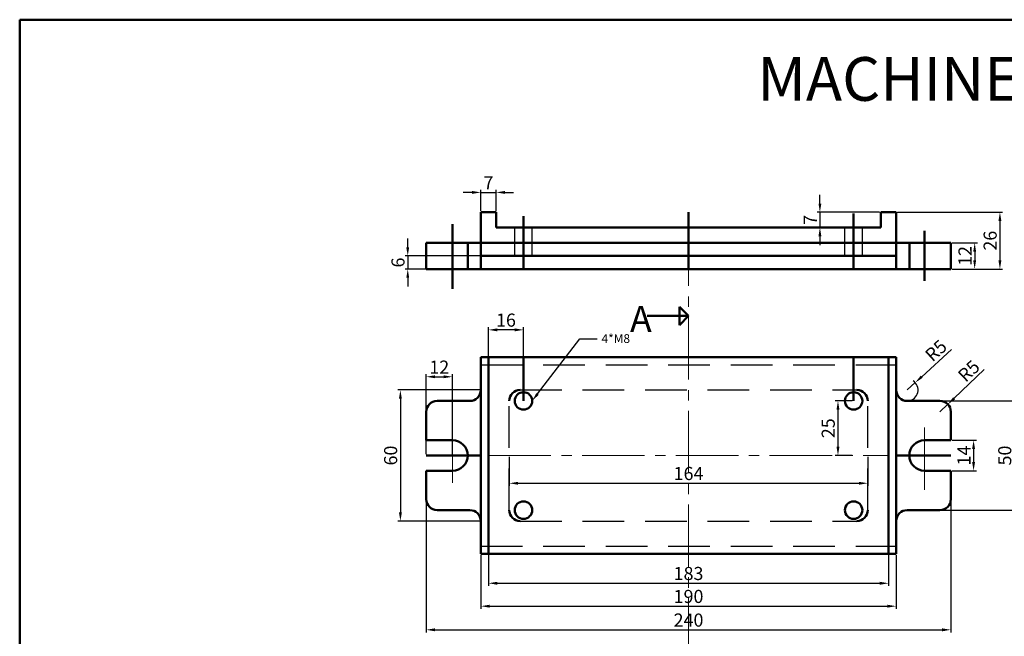
# Model space of a CAD drawing. Units: millimetres. Extents: x -1209 to -333, y 66 to 707.
# Tile 2 of 4: x -1209 to -759, y 424 to 707. Entities that reach past the tile are written whole.
import ezdxf
from ezdxf import colors
from ezdxf.entities.mleader import LeaderData, LeaderLine
from ezdxf.math import Vec2, Vec3

# ---------------------------------------------------------------- set-up
doc = ezdxf.new("R2010")
doc.units = ezdxf.units.MM
doc.header["$LTSCALE"] = 1.5
doc.linetypes.add('CENTER2', pattern=[28.575, 19.05, -3.175, 3.175, -3.175])
doc.linetypes.add('DASHED', pattern=[19.05, 12.7, -6.35])
for name, color, linetype, lineweight in [('M-CNTR', 1, 'CENTER2', 18), ('M-DIMS', 2, 'Continuous', 25), ('M-HIDN', 4, 'DASHED', 25), ('M-OUTL', 7, 'Continuous', 50), ('M-TEXT', 3, 'Continuous', 25), ('M-TTLB', 7, 'Continuous', 50)]:
    doc.layers.add(name, color=color, linetype=linetype, lineweight=lineweight)
doc.styles.get("Standard").update_dxf_attribs({"font": 'arial.ttf'})
doc.dimstyles.new('ISO-25', dxfattribs={"dimtxt": 6, "dimasz": 4, "dimexe": 1.25, "dimexo": 0.625, "dimtad": 1, "dimdec": 0, "dimtxsty": 'Standard', "dimcen": 2.5, "dimadec": 0, "dimazin": 0, "dimtfac": 1, "dimtdec": 0, "dimtmove": 0, "dimatfit": 3, "dimfxl": 1, "dimarcsym": 0})

# ---------------------------------------------------------------- blocks, each defined once
blk = doc.blocks.new('*D1')
at = {"layer": 'Defpoints', "color": 0, "transparency": 16777216}
for p in [(-998.18, 462.21), (-808.18, 462.21), (-808.18, 438.24)]:
    blk.add_point(p, dxfattribs=at)
at = {"layer": 'M-DIMS', "color": 0, "lineweight": -2, "transparency": 16777216}
for p, q in [((-998.18, 461.59), (-998.18, 436.99)), ((-808.18, 461.59), (-808.18, 436.99)), ((-994.18, 438.24), (-812.18, 438.24))]:
    blk.add_line(p, q, dxfattribs=at)
at = {"layer": 'M-DIMS', "color": 0, "transparency": 16777216}
for points in [[(-994.18, 438.9), (-994.18, 437.57), (-998.18, 438.24)], [(-812.18, 438.9), (-812.18, 437.57), (-808.18, 438.24)]]:
    blk.add_solid(points, dxfattribs=at)
at = {"layer": 'M-DIMS', "color": 0, "transparency": 16777216, "insert": (-903.18, 441.93), "char_height": 6, "attachment_point": 5}
blk.add_mtext('190', dxfattribs=at)
blk = doc.blocks.new('*D2')
at = {"layer": 'Defpoints', "color": 0, "transparency": 16777216}
for p in [(-994.68, 465.71), (-811.68, 465.71), (-811.68, 448.73)]:
    blk.add_point(p, dxfattribs=at)
at = {"layer": 'M-DIMS', "color": 0, "lineweight": -2, "transparency": 16777216}
for p, q in [((-994.68, 465.09), (-994.68, 447.48)), ((-811.68, 465.09), (-811.68, 447.48)), ((-990.68, 448.73), (-815.68, 448.73))]:
    blk.add_line(p, q, dxfattribs=at)
at = {"layer": 'M-DIMS', "color": 0, "transparency": 16777216}
for points in [[(-990.68, 449.39), (-990.68, 448.06), (-994.68, 448.73)], [(-815.68, 449.39), (-815.68, 448.06), (-811.68, 448.73)]]:
    blk.add_solid(points, dxfattribs=at)
at = {"layer": 'M-DIMS', "color": 0, "transparency": 16777216, "insert": (-903.18, 452.42), "char_height": 6, "attachment_point": 5}
blk.add_mtext('183', dxfattribs=at)
blk = doc.blocks.new('*D3')
at = {"layer": 'Defpoints', "color": 0, "transparency": 16777216}
for p in [(-1023.18, 487.21), (-783.18, 487.21), (-783.18, 427.42)]:
    blk.add_point(p, dxfattribs=at)
at = {"layer": 'M-DIMS', "color": 0, "lineweight": -2, "transparency": 16777216}
for p, q in [((-1023.18, 486.59), (-1023.18, 426.17)), ((-783.18, 486.59), (-783.18, 426.17)), ((-1019.18, 427.42), (-787.18, 427.42))]:
    blk.add_line(p, q, dxfattribs=at)
at = {"layer": 'M-DIMS', "color": 0, "transparency": 16777216}
for points in [[(-1019.18, 428.09), (-1019.18, 426.75), (-1023.18, 427.42)], [(-787.18, 428.09), (-787.18, 426.75), (-783.18, 427.42)]]:
    blk.add_solid(points, dxfattribs=at)
at = {"layer": 'M-DIMS', "color": 0, "transparency": 16777216, "insert": (-903.18, 431.11), "char_height": 6, "attachment_point": 5}
blk.add_mtext('240', dxfattribs=at)
blk = doc.blocks.new('*D4')
at = {"layer": 'Defpoints', "color": 0, "transparency": 16777216}
for p in [(-998.18, 537.21), (-1034.96, 477.21), (-998.18, 477.21)]:
    blk.add_point(p, dxfattribs=at)
at = {"layer": 'M-DIMS', "color": 0, "lineweight": -2, "transparency": 16777216}
for p, q in [((-998.81, 537.21), (-1036.21, 537.21)), ((-1034.96, 533.21), (-1034.96, 481.21)), ((-998.81, 477.21), (-1036.21, 477.21))]:
    blk.add_line(p, q, dxfattribs=at)
at = {"layer": 'M-DIMS', "color": 0, "transparency": 16777216}
for points in [[(-1035.62, 533.21), (-1034.29, 533.21), (-1034.96, 537.21)], [(-1035.62, 481.21), (-1034.29, 481.21), (-1034.96, 477.21)]]:
    blk.add_solid(points, dxfattribs=at)
at = {"layer": 'M-DIMS', "color": 0, "transparency": 16777216, "insert": (-1038.65, 507.21), "char_height": 6, "attachment_point": 5, "rotation": 90}
blk.add_mtext('60', dxfattribs=at)
blk = doc.blocks.new('*D5')
at = {"layer": 'Defpoints', "color": 0, "transparency": 16777216}
for p in [(-788.18, 532.21), (-788.18, 482.21), (-754.08, 482.21)]:
    blk.add_point(p, dxfattribs=at)
at = {"layer": 'M-DIMS', "color": 0, "lineweight": -2, "transparency": 16777216}
for p, q in [((-787.56, 532.21), (-752.83, 532.21)), ((-754.08, 528.21), (-754.08, 486.21)), ((-787.56, 482.21), (-752.83, 482.21))]:
    blk.add_line(p, q, dxfattribs=at)
at = {"layer": 'M-DIMS', "color": 0, "transparency": 16777216}
for points in [[(-754.75, 528.21), (-753.41, 528.21), (-754.08, 532.21)], [(-754.75, 486.21), (-753.41, 486.21), (-754.08, 482.21)]]:
    blk.add_solid(points, dxfattribs=at)
at = {"layer": 'M-DIMS', "color": 0, "transparency": 16777216, "insert": (-757.77, 507.21), "char_height": 6, "attachment_point": 5, "rotation": 90}
blk.add_mtext('50', dxfattribs=at)
blk = doc.blocks.new('*D6')
at = {"layer": 'Defpoints', "color": 0, "transparency": 16777216}
for p in [(-783.18, 514.21), (-783.18, 500.21), (-772.79, 500.21)]:
    blk.add_point(p, dxfattribs=at)
at = {"layer": 'M-DIMS', "color": 0, "lineweight": -2, "transparency": 16777216}
for p, q in [((-782.56, 514.21), (-771.54, 514.21)), ((-772.79, 510.21), (-772.79, 504.21)), ((-782.56, 500.21), (-771.54, 500.21))]:
    blk.add_line(p, q, dxfattribs=at)
at = {"layer": 'M-DIMS', "color": 0, "transparency": 16777216}
for points in [[(-773.46, 510.21), (-772.13, 510.21), (-772.79, 514.21)], [(-773.46, 504.21), (-772.13, 504.21), (-772.79, 500.21)]]:
    blk.add_solid(points, dxfattribs=at)
at = {"layer": 'M-DIMS', "color": 0, "transparency": 16777216, "insert": (-776.43, 507.21), "char_height": 6, "attachment_point": 5, "rotation": 90}
blk.add_mtext('14', dxfattribs=at)
blk = doc.blocks.new('*D7')
at = {"layer": 'Defpoints', "color": 0, "transparency": 16777216}
for p in [(-788.18, 527.21), (-784.56, 530.66)]:
    blk.add_point(p, dxfattribs=at)
at = {"layer": 'M-DIMS', "color": 0, "lineweight": -2, "transparency": 16777216}
for p, q in [((-767.92, 546.52), (-781.67, 533.42)), ((-788.18, 527.21), (-784.56, 530.66))]:
    blk.add_line(p, q, dxfattribs=at)
at = {"layer": 'M-DIMS', "color": 0, "transparency": 16777216}
blk.add_solid([(-782.13, 533.9), (-781.21, 532.94), (-784.56, 530.66)], dxfattribs=at)
at = {"layer": 'M-DIMS', "color": 0, "transparency": 16777216, "insert": (-774.43, 545.39), "char_height": 6, "attachment_point": 5, "rotation": 43.6176}
blk.add_mtext('R5', dxfattribs=at)
blk = doc.blocks.new('*D8')
at = {"layer": 'Defpoints', "color": 0, "transparency": 16777216}
for p in [(-799.49, 540.58), (-803.18, 537.21)]:
    blk.add_point(p, dxfattribs=at)
at = {"layer": 'M-DIMS', "color": 0, "lineweight": -2, "transparency": 16777216}
for p, q in [((-782.95, 555.67), (-796.53, 543.28)), ((-803.18, 537.21), (-799.49, 540.58))]:
    blk.add_line(p, q, dxfattribs=at)
blk.add_arc((-803.18, 537.21), 5, 277.162, 56.6885, dxfattribs=at)
at = {"layer": 'M-DIMS', "color": 0, "transparency": 16777216}
blk.add_solid([(-796.98, 543.77), (-796.08, 542.78), (-799.49, 540.58)], dxfattribs=at)
at = {"layer": 'M-DIMS', "color": 0, "transparency": 16777216, "insert": (-789.48, 554.69), "char_height": 6, "attachment_point": 5, "rotation": 42.3646}
blk.add_mtext('R5', dxfattribs=at)
blk = doc.blocks.new('*D9')
at = {"layer": 'Defpoints', "color": 0, "transparency": 16777216}
for p in [(-827.68, 532.21), (-834.82, 507.21), (-827.68, 507.21)]:
    blk.add_point(p, dxfattribs=at)
at = {"layer": 'M-DIMS', "color": 0, "lineweight": -2, "transparency": 16777216}
for p, q in [((-828.31, 532.21), (-836.07, 532.21)), ((-834.82, 528.21), (-834.82, 511.21)), ((-828.31, 507.21), (-836.07, 507.21))]:
    blk.add_line(p, q, dxfattribs=at)
at = {"layer": 'M-DIMS', "color": 0, "transparency": 16777216}
for points in [[(-835.49, 528.21), (-834.16, 528.21), (-834.82, 532.21)], [(-835.49, 511.21), (-834.16, 511.21), (-834.82, 507.21)]]:
    blk.add_solid(points, dxfattribs=at)
at = {"layer": 'M-DIMS', "color": 0, "transparency": 16777216, "insert": (-838.51, 519.71), "char_height": 6, "attachment_point": 5, "rotation": 90}
blk.add_mtext('25', dxfattribs=at)
blk = doc.blocks.new('*D10')
at = {"layer": 'Defpoints', "color": 0, "transparency": 16777216}
for p in [(-985.18, 507.21), (-821.18, 507.21), (-821.18, 494.51)]:
    blk.add_point(p, dxfattribs=at)
at = {"layer": 'M-DIMS', "color": 0, "lineweight": -2, "transparency": 16777216}
for p, q in [((-985.18, 506.59), (-985.18, 493.26)), ((-821.18, 506.59), (-821.18, 493.26)), ((-981.18, 494.51), (-825.18, 494.51))]:
    blk.add_line(p, q, dxfattribs=at)
at = {"layer": 'M-DIMS', "color": 0, "transparency": 16777216}
for points in [[(-981.18, 495.17), (-981.18, 493.84), (-985.18, 494.51)], [(-825.18, 495.17), (-825.18, 493.84), (-821.18, 494.51)]]:
    blk.add_solid(points, dxfattribs=at)
at = {"layer": 'M-DIMS', "color": 0, "transparency": 16777216, "insert": (-903.18, 498.19), "char_height": 6, "attachment_point": 5}
blk.add_mtext('164', dxfattribs=at)
blk = doc.blocks.new('*D11')
at = {"layer": 'Defpoints', "color": 0, "transparency": 16777216}
for p in [(-1011.18, 543.26), (-1023.18, 507.21), (-1011.18, 507.21)]:
    blk.add_point(p, dxfattribs=at)
at = {"layer": 'M-DIMS', "color": 0, "lineweight": -2, "transparency": 16777216}
for p, q in [((-1023.18, 507.84), (-1023.18, 544.51)), ((-1019.18, 543.26), (-1015.18, 543.26)), ((-1011.18, 507.84), (-1011.18, 544.51))]:
    blk.add_line(p, q, dxfattribs=at)
at = {"layer": 'M-DIMS', "color": 0, "transparency": 16777216}
for points in [[(-1019.18, 543.92), (-1019.18, 542.59), (-1023.18, 543.26)], [(-1015.18, 543.92), (-1015.18, 542.59), (-1011.18, 543.26)]]:
    blk.add_solid(points, dxfattribs=at)
at = {"layer": 'M-DIMS', "color": 0, "transparency": 16777216, "insert": (-1017.18, 546.89), "char_height": 6, "attachment_point": 5}
blk.add_mtext('12', dxfattribs=at)
blk = doc.blocks.new('*D12')
at = {"layer": 'Defpoints', "color": 0, "transparency": 16777216}
for p in [(-994.68, 564.73), (-994.68, 532.21), (-978.68, 532.21)]:
    blk.add_point(p, dxfattribs=at)
at = {"layer": 'M-DIMS', "color": 0, "lineweight": -2, "transparency": 16777216}
for p, q in [((-994.68, 532.84), (-994.68, 565.98)), ((-982.68, 564.73), (-990.68, 564.73)), ((-978.68, 532.84), (-978.68, 565.98))]:
    blk.add_line(p, q, dxfattribs=at)
at = {"layer": 'M-DIMS', "color": 0, "transparency": 16777216}
for points in [[(-990.68, 565.4), (-990.68, 564.07), (-994.68, 564.73)], [(-982.68, 565.4), (-982.68, 564.07), (-978.68, 564.73)]]:
    blk.add_solid(points, dxfattribs=at)
at = {"layer": 'M-DIMS', "color": 0, "transparency": 16777216, "insert": (-986.68, 568.42), "char_height": 6, "attachment_point": 5}
blk.add_mtext('16', dxfattribs=at)
blk = doc.blocks.new('*D13')
at = {"layer": 'Defpoints', "color": 0, "transparency": 16777216}
for p in [(-783.18, 604.56), (-783.18, 592.56), (-772.3, 592.56)]:
    blk.add_point(p, dxfattribs=at)
at = {"layer": 'M-DIMS', "color": 0, "lineweight": -2, "transparency": 16777216}
for p, q in [((-782.56, 604.56), (-771.05, 604.56)), ((-772.3, 600.56), (-772.3, 596.56)), ((-782.56, 592.56), (-771.05, 592.56))]:
    blk.add_line(p, q, dxfattribs=at)
at = {"layer": 'M-DIMS', "color": 0, "transparency": 16777216}
for points in [[(-772.97, 600.56), (-771.64, 600.56), (-772.3, 604.56)], [(-772.97, 596.56), (-771.64, 596.56), (-772.3, 592.56)]]:
    blk.add_solid(points, dxfattribs=at)
at = {"layer": 'M-DIMS', "color": 0, "transparency": 16777216, "insert": (-775.94, 598.56), "char_height": 6, "attachment_point": 5, "rotation": 90}
blk.add_mtext('12', dxfattribs=at)
blk = doc.blocks.new('*D14')
at = {"layer": 'Defpoints', "color": 0, "transparency": 16777216}
for p in [(-808.18, 618.56), (-783.18, 592.56), (-760.75, 592.56)]:
    blk.add_point(p, dxfattribs=at)
at = {"layer": 'M-DIMS', "color": 0, "lineweight": -2, "transparency": 16777216}
for p, q in [((-807.56, 618.56), (-759.5, 618.56)), ((-760.75, 614.56), (-760.75, 596.56)), ((-782.56, 592.56), (-759.5, 592.56))]:
    blk.add_line(p, q, dxfattribs=at)
at = {"layer": 'M-DIMS', "color": 0, "transparency": 16777216}
for points in [[(-761.42, 614.56), (-760.08, 614.56), (-760.75, 618.56)], [(-761.42, 596.56), (-760.08, 596.56), (-760.75, 592.56)]]:
    blk.add_solid(points, dxfattribs=at)
at = {"layer": 'M-DIMS', "color": 0, "transparency": 16777216, "insert": (-764.44, 605.56), "char_height": 6, "attachment_point": 5, "rotation": 90}
blk.add_mtext('26', dxfattribs=at)
blk = doc.blocks.new('*D15')
at = {"layer": 'Defpoints', "color": 0, "transparency": 16777216}
for p in [(-815.16, 618.56), (-843.09, 611.56), (-815.16, 611.56)]:
    blk.add_point(p, dxfattribs=at)
at = {"layer": 'M-DIMS', "color": 0, "lineweight": -2, "transparency": 16777216}
for p, q in [((-843.09, 622.56), (-843.09, 626.56)), ((-815.78, 618.56), (-844.34, 618.56)), ((-843.09, 618.56), (-843.09, 611.56)), ((-815.78, 611.56), (-844.34, 611.56)), ((-843.09, 607.56), (-843.09, 603.56))]:
    blk.add_line(p, q, dxfattribs=at)
at = {"layer": 'M-DIMS', "color": 0, "transparency": 16777216}
for points in [[(-843.75, 622.56), (-842.42, 622.56), (-843.09, 618.56)], [(-843.75, 607.56), (-842.42, 607.56), (-843.09, 611.56)]]:
    blk.add_solid(points, dxfattribs=at)
at = {"layer": 'M-DIMS', "color": 0, "transparency": 16777216, "insert": (-846.71, 615.06), "char_height": 6, "attachment_point": 5, "rotation": 90}
blk.add_mtext('7', dxfattribs=at)
blk = doc.blocks.new('*D16')
at = {"layer": 'Defpoints', "color": 0, "transparency": 16777216}
for p in [(-991.18, 627.65), (-998.18, 618.56), (-991.18, 618.56)]:
    blk.add_point(p, dxfattribs=at)
at = {"layer": 'M-DIMS', "color": 0, "lineweight": -2, "transparency": 16777216}
for p, q in [((-1002.18, 627.65), (-1006.18, 627.65)), ((-998.18, 619.19), (-998.18, 628.9)), ((-998.18, 627.65), (-991.18, 627.65)), ((-991.18, 619.19), (-991.18, 628.9)), ((-987.18, 627.65), (-983.18, 627.65))]:
    blk.add_line(p, q, dxfattribs=at)
at = {"layer": 'M-DIMS', "color": 0, "transparency": 16777216}
for points in [[(-1002.18, 628.31), (-1002.18, 626.98), (-998.18, 627.65)], [(-987.18, 628.31), (-987.18, 626.98), (-991.18, 627.65)]]:
    blk.add_solid(points, dxfattribs=at)
at = {"layer": 'M-DIMS', "color": 0, "transparency": 16777216, "insert": (-994.68, 631.27), "char_height": 6, "attachment_point": 5}
blk.add_mtext('7', dxfattribs=at)
blk = doc.blocks.new('*D17')
at = {"layer": 'Defpoints', "color": 0, "transparency": 16777216}
for p in [(-978.68, 598.56), (-1031.6, 592.56), (-978.68, 592.56)]:
    blk.add_point(p, dxfattribs=at)
at = {"layer": 'M-DIMS', "color": 0, "lineweight": -2, "transparency": 16777216}
for p, q in [((-1031.6, 602.56), (-1031.6, 606.56)), ((-979.31, 598.56), (-1032.85, 598.56)), ((-1031.6, 598.56), (-1031.6, 592.56)), ((-979.31, 592.56), (-1032.85, 592.56)), ((-1031.6, 588.56), (-1031.6, 584.56))]:
    blk.add_line(p, q, dxfattribs=at)
at = {"layer": 'M-DIMS', "color": 0, "transparency": 16777216}
for points in [[(-1032.27, 602.56), (-1030.94, 602.56), (-1031.6, 598.56)], [(-1032.27, 588.56), (-1030.94, 588.56), (-1031.6, 592.56)]]:
    blk.add_solid(points, dxfattribs=at)
at = {"layer": 'M-DIMS', "color": 0, "transparency": 16777216, "insert": (-1035.29, 595.56), "char_height": 6, "attachment_point": 5, "rotation": 90}
blk.add_mtext('6', dxfattribs=at)

msp = doc.modelspace()

# ---------------------------------------------------------------- linework, layer by layer
at = {"layer": 'M-CNTR'}
for p, q in [((-903.18, 413.37), (-903.18, 617.86)), ((-1011.18, 494.66), (-1011.18, 518.08)), ((-795.18, 491.51), (-795.18, 520.41)), ((-994.68, 507.21), (-811.68, 507.21))]:
    msp.add_line(p, q, dxfattribs=at)
at = {"layer": 'M-HIDN'}
for p, q in [((-982.68, 598.56), (-982.68, 611.56)), ((-974.68, 598.56), (-974.68, 611.56)), ((-831.68, 598.56), (-831.68, 611.56)), ((-823.68, 598.56), (-823.68, 611.56)), ((-998.18, 548.71), (-808.18, 548.71)), ((-980.18, 537.21), (-826.18, 537.21)), ((-985.18, 482.21), (-985.18, 532.21)), ((-821.18, 482.21), (-821.18, 532.21)), ((-980.18, 477.21), (-826.18, 477.21)), ((-998.18, 465.71), (-808.18, 465.71))]:
    msp.add_line(p, q, dxfattribs=at)
at = {"layer": 'M-OUTL'}
for p, q in [((-998.18, 592.56), (-998.18, 618.56)), ((-991.18, 618.56), (-998.18, 618.56)), ((-991.18, 611.56), (-991.18, 618.56)), ((-903.18, 592.56), (-903.18, 618.56)), ((-827.68, 592.56), (-827.68, 617.94)), ((-808.18, 618.56), (-815.16, 618.56)), ((-815.16, 611.56), (-815.16, 618.56)), ((-808.18, 592.56), (-808.18, 618.56)), ((-1011.18, 583.49), (-1011.18, 613.17)), ((-978.68, 592.56), (-978.68, 616.84)), ((-815.16, 611.56), (-991.18, 611.56)), ((-795.18, 610.06), (-795.18, 587.16)), ((-1023.18, 592.56), (-1023.18, 604.56)), ((-1023.18, 604.56), (-783.18, 604.56)), ((-1004.18, 592.56), (-1004.18, 604.56)), ((-802.18, 604.56), (-802.18, 592.56)), ((-783.18, 604.56), (-783.18, 592.56)), ((-998.18, 598.56), (-808.18, 598.56)), ((-783.18, 592.56), (-1023.18, 592.56)), ((-903.18, 592.56), (-783.18, 592.56)), ((-998.18, 552.21), (-808.18, 552.21)), ((-998.18, 462.21), (-998.18, 552.21)), ((-994.68, 462.21), (-994.68, 552.21)), ((-978.68, 532.21), (-978.68, 552.21)), ((-827.68, 532.21), (-827.68, 552.21)), ((-811.68, 462.21), (-811.68, 552.21)), ((-808.18, 462.21), (-808.18, 552.21)), ((-1018.18, 532.21), (-1003.18, 532.21)), ((-803.18, 532.21), (-788.18, 532.21)), ((-1023.18, 514.21), (-1023.18, 527.21)), ((-783.18, 514.21), (-783.18, 527.21)), ((-1023.18, 514.21), (-1011.18, 514.21)), ((-795.18, 514.21), (-783.18, 514.21)), ((-1023.18, 507.21), (-998.18, 507.21)), ((-808.18, 507.21), (-783.18, 507.21)), ((-1023.18, 487.21), (-1023.18, 500.21)), ((-1023.18, 500.21), (-1011.18, 500.21)), ((-795.18, 500.21), (-783.18, 500.21)), ((-783.18, 487.21), (-783.18, 500.21)), ((-1018.18, 482.21), (-1003.18, 482.21)), ((-803.18, 482.21), (-788.18, 482.21)), ((-998.18, 462.21), (-808.18, 462.21))]:
    msp.add_line(p, q, dxfattribs=at)
at = {"layer": 'M-OUTL', "ltscale": 0.4}
for p, q in [((-903.18, 571.14), (-907.36, 575.32)), ((-907.36, 575.32), (-907.36, 566.95)), ((-903.18, 571.14), (-922.06, 571.14)), ((-903.18, 571.14), (-907.36, 566.95))]:
    msp.add_line(p, q, dxfattribs=at)
at = {"layer": 'M-OUTL'}
for centre in [(-978.68, 532.21), (-827.68, 532.21), (-978.68, 482.21), (-827.68, 482.21)]:
    msp.add_circle(centre, 4, dxfattribs=at)
for centre, radius, start, end in [((-1003.18, 537.21), 5, 270, 0), ((-980.18, 532.21), 5, 90, 180), ((-826.18, 532.21), 5, 0, 90), ((-803.18, 537.21), 5, 180, 270), ((-1018.18, 527.21), 5, 90, 180), ((-788.18, 527.21), 5, 0, 90), ((-1011.18, 507.21), 7, 270, 90), ((-795.18, 507.21), 7, 90, 270), ((-1018.18, 487.21), 5, 180, 270), ((-788.18, 487.21), 5, 270, 0), ((-1003.18, 477.21), 5, 0, 90), ((-980.18, 482.21), 5, 180, 270), ((-826.18, 482.21), 5, 270, 0), ((-803.18, 477.21), 5, 90, 180)]:
    msp.add_arc(centre, radius, start, end, dxfattribs=at)
at = {"layer": 'M-TTLB', "ltscale": 0.4}
msp.add_lwpolyline([(-1209.09, 706.73), (-332.54, 706.73), (-332.54, 66.01), (-1209.09, 66.01)], close=True, dxfattribs=at)

# ---------------------------------------------------------------- texts
at = {"layer": 'M-TEXT', "ltscale": 0.4, "attachment_point": 1}
for s, width, insert, char_height in [('\\pxqc;MACHINE VICE', 213.0298, (-886.63, 689.59), 20), ('A', 7.4448, (-929.96, 575.73), 12)]:
    msp.add_mtext_dynamic_manual_height_columns(s, width=width, gutter_width=12.5, heights=[0], dxfattribs=dict(at, insert=insert, char_height=char_height))

# ---------------------------------------------------------------- dimensions: what is measured, and where the dimension line sits
at = {"layer": 'M-DIMS'}
for base, p1, p2, picture, middle in [((-991.18, 627.65), (-998.18, 618.56), (-991.18, 618.56), '*D16', (-994.68, 631.27)), ((-994.68, 564.73), (-978.68, 532.21), (-994.68, 532.21), '*D12', (-986.68, 568.42)), ((-1011.18, 543.26), (-1023.18, 507.21), (-1011.18, 507.21), '*D11', (-1017.18, 546.89)), ((-821.18, 494.51), (-985.18, 507.21), (-821.18, 507.21), '*D10', (-903.18, 498.19)), ((-783.18, 427.42), (-1023.18, 487.21), (-783.18, 487.21), '*D3', (-903.18, 431.11)), ((-811.68, 448.73), (-994.68, 465.71), (-811.68, 465.71), '*D2', (-903.18, 452.42)), ((-808.18, 438.24), (-998.18, 462.21), (-808.18, 462.21), '*D1', (-903.18, 441.93))]:
    dim = msp.add_linear_dim(base=base, p1=p1, p2=p2, dimstyle='ISO-25', override={"dimclrd": 0, "dimclre": 0, "dimclrt": 0}, dxfattribs=at)
    dim.commit()
    dim.dimension.update_dxf_attribs({"geometry": picture, "text_midpoint": middle})
for base, p1, p2, picture, middle in [((-843.09, 611.56), (-815.16, 618.56), (-815.16, 611.56), '*D15', (-846.71, 615.06)), ((-760.75, 592.56), (-808.18, 618.56), (-783.18, 592.56), '*D14', (-764.44, 605.56)), ((-1031.6, 592.56), (-978.68, 598.56), (-978.68, 592.56), '*D17', (-1035.29, 595.56)), ((-772.3, 592.56), (-783.18, 604.56), (-783.18, 592.56), '*D13', (-775.94, 598.56)), ((-1034.96, 477.21), (-998.18, 537.21), (-998.18, 477.21), '*D4', (-1038.65, 507.21)), ((-834.82, 507.21), (-827.68, 532.21), (-827.68, 507.21), '*D9', (-838.51, 519.71)), ((-754.08, 482.21), (-788.18, 532.21), (-788.18, 482.21), '*D5', (-757.77, 507.21)), ((-772.79, 500.21), (-783.18, 514.21), (-783.18, 500.21), '*D6', (-776.43, 507.21))]:
    dim = msp.add_linear_dim(base=base, p1=p1, p2=p2, angle=90, dimstyle='ISO-25', override={"dimclrd": 0, "dimclre": 0, "dimclrt": 0}, dxfattribs=at)
    dim.commit()
    dim.dimension.update_dxf_attribs({"geometry": picture, "text_midpoint": middle})
for center, mpoint, picture, middle in [((-803.18, 537.21), (-799.49, 540.58), '*D8', (-787, 551.97)), ((-788.18, 527.21), (-784.56, 530.66), '*D7', (-771.89, 542.73))]:
    dim = msp.add_radius_dim(center=center, mpoint=mpoint, dimstyle='ISO-25', override={"dimclrd": 0, "dimclre": 0, "dimclrt": 0}, dxfattribs=at)
    dim.commit()
    dim.dimension.update_dxf_attribs({"geometry": picture, "text_midpoint": middle, "dimtype": 164})

# ---------------------------------------------------------------- leaders
at = {"layer": 'M-DIMS', "ltscale": 0.4}
ml = msp.add_multileader_mtext('Standard', dxfattribs=at)
ml.set_content('4*M8', color=256)
ml.set_leader_properties()
ml.build(insert=Vec2(0, 0))
ctx = ml.context
ctx.base_point, ctx.plane_origin = Vec3(-944.96, 560.7), Vec3(-974.68, 532.21)
notes = []
notes.append((ctx, [(0, (1, 1, 0), (-952.96, 560.7), (1, 0), 8, [(0, [(-974.68, 532.21)], 0, [])])]))
ctx.mtext.insert, ctx.mtext.flow_direction = Vec3(-942.96, 562.74), 5
for ctx, leaders in notes:
    for number, flags, end, landing, length, lines in leaders:
        leader = LeaderData()
        leader.index, (leader.has_last_leader_line, leader.has_dogleg_vector, leader.attachment_direction) = number, flags
        leader.last_leader_point, leader.dogleg_vector, leader.dogleg_length = Vec3(end), Vec3(landing), length
        for number, points, colour, breaks in lines:
            line = LeaderLine()
            line.index, line.vertices, line.color, line.breaks = number, Vec3.list(points), colors.encode_raw_color(colour), breaks
            leader.lines.append(line)
        ctx.leaders.append(leader)

doc.saveas('drawing.dxf')
